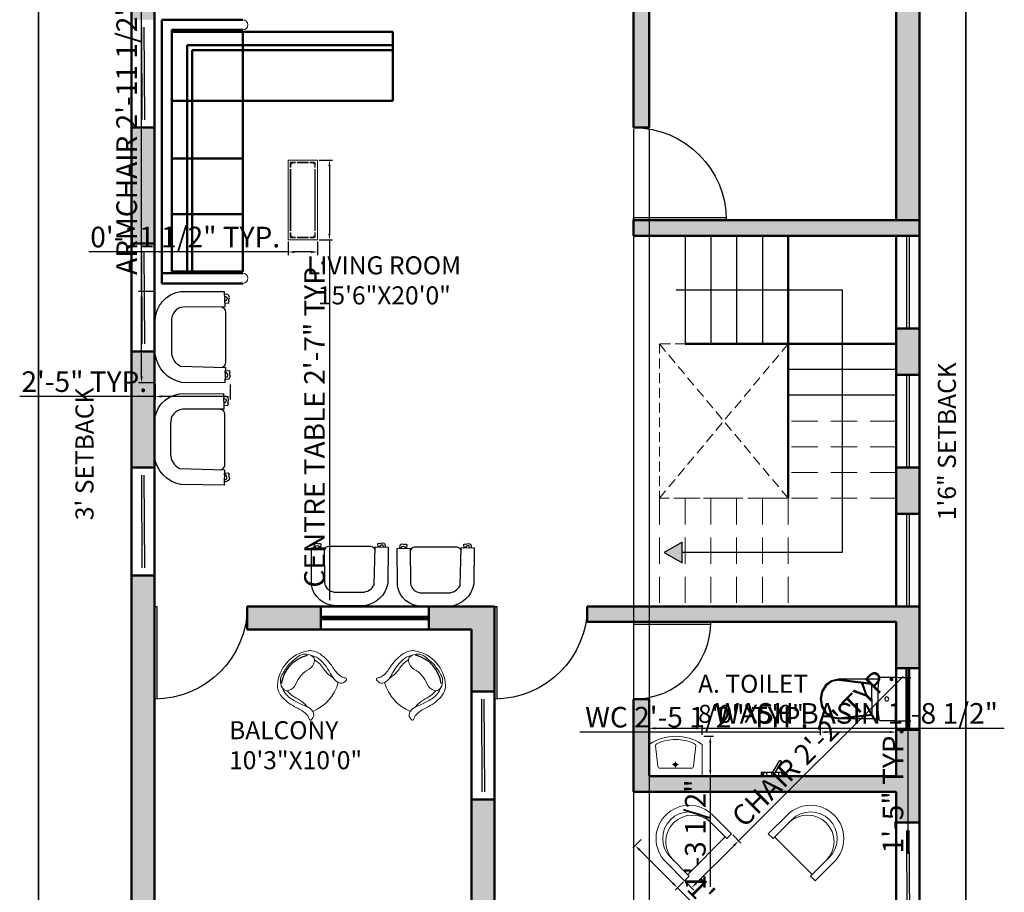
# Model space of a CAD drawing. Units: inches. Extents: x 1986 to 21484, y -1816 to 2016.
# Tile 42 of 85: x 2493 to 2875, y 1277 to 1616. Entities that reach past the tile are written whole.
import ezdxf

# ---------------------------------------------------------------- set-up
doc = ezdxf.new("R2010")
doc.units = ezdxf.units.IN
doc.linetypes.add('DASHED', pattern=[19.05, 12.7, -6.35])
for name, color, linetype in [('2D', 7, 'Continuous'), ('IFF-FURN-DETAIL', 250, 'Continuous'), ('SANTEH', 7, 'Continuous')]:
    doc.layers.add(name, color=color, linetype=linetype)
for name, color, linetype, lineweight in [('A-ANNO-DIMS', 2, 'Continuous', 18), ('A-ANNO-TEXT', 7, 'Continuous', 18), ('A-AREA-IDEN', 3, 'Continuous', 18), ('A-DOOR', 3, 'Continuous', 25), ('A-FLOR-FIXT', 8, 'Continuous', 18), ('A-FLOR-STRS', 7, 'Continuous', 25), ('A-FLOR-STRS-OVHD', 8, 'DASHED', 18), ('A-FURN', 8, 'Continuous', 18), ('A-GLAZ', 4, 'Continuous', 25), ('A-WALL', 7, 'Continuous', 50), ('A-WALL-PATT', 8, 'Continuous', 13), ('C-PROP', 7, 'Continuous', 35)]:
    doc.layers.add(name, color=color, linetype=linetype, lineweight=lineweight)
doc.styles.get("Standard").update_dxf_attribs({"font": 'arial.ttf'})
doc.dimstyles.new('ISO-25', dxfattribs={"dimtxt": 8, "dimasz": 2.5, "dimexe": 1.25, "dimexo": 0.625, "dimtad": 1, "dimdec": 1, "dimlunit": 3, "dimtxsty": 'Standard', "dimcen": 2.5, "dimadec": 0, "dimazin": 0, "dimtfac": 1, "dimtdec": 1, "dimtmove": 0, "dimatfit": 3, "dimfxl": 1, "dimarcsym": 0})

# ---------------------------------------------------------------- blocks, each defined once
blk = doc.blocks.new('D1')
for p, q in [((1805.96, 1500.36), (1805.96, 1464.36)), ((1806.96, 1500.36), (1806.96, 1464.36)), ((1805.96, 1464.36), (1806.96, 1464.36))]:
    blk.add_line(p, q)
blk.add_arc((1805.96, 1464.36), 36, 0, 90)
blk = doc.blocks.new('D2')
for p, q in [((1722.5, 1505.46), (1722.5, 1475.46)), ((1723.5, 1505.46), (1723.5, 1475.46)), ((1722.5, 1475.46), (1723.5, 1475.46))]:
    blk.add_line(p, q)
blk.add_arc((1722.5, 1475.46), 30, 0, 90)
blk = doc.blocks.new('WC 2 Symb_109')
at = {"layer": 'SANTEH'}
for p, q in [((0, 0), (0, 380)), ((0, 380), (132.4, 380)), ((153.6, 364.9), (506.8, 364.9)), ((506.3, 364.9), (215.7, 330.9)), ((506.3, 356), (215.7, 322)), ((215.7, 190), (215.7, 330.9)), ((215.7, 190), (215.7, 49.1)), ((153.8, 15.1), (506.8, 15.1)), ((506.3, 24), (215.7, 58)), ((506.3, 15.1), (215.7, 49.1)), ((0, 0), (132.4, 0))]:
    blk.add_line(p, q, dxfattribs=at)
for points in [[(154.6, 360.1), (153.9, 364.1), (152.3, 367.9), (150.2, 371.3), (147.4, 374.3), (144.1, 376.7), (140.5, 378.5), (136.5, 379.6), (132.4, 380)], [(154.6, 19.7), (158.6, 62.1), (161.4, 104.7), (163.1, 147.3), (163.7, 189.9), (163.1, 232.5), (161.4, 275.1), (158.6, 317.7), (154.6, 360.1)], [(506.3, 24), (565.5, 36.6), (615.7, 72.6), (649.2, 126.5), (661, 190), (649.2, 253.5), (615.7, 307.4), (565.5, 343.4), (506.3, 356)], [(506.8, 15.1), (569.2, 28.4), (622.2, 66.3), (657.6, 123.1), (670, 190), (657.6, 256.9), (622.2, 313.7), (569.2, 351.6), (506.8, 364.9)], [(132.4, 0), (136.5, 0.4), (140.4, 1.5), (144.1, 3.2), (147.3, 5.6), (150.1, 8.6), (152.3, 12), (153.8, 15.7), (154.6, 19.7)]]:
    blk.add_lwpolyline(points, dxfattribs=at)
blk.add_lwpolyline([(83.6, 208.5), (70.4, 203.1), (64.9, 190), (70.4, 176.9), (83.6, 171.5), (96.8, 176.9), (102.2, 190), (96.8, 203.1)], close=True, dxfattribs=at)
blk = doc.blocks.new('A$C2EBB240D')
for p, q in [((480, 375.8), (20, 375.8)), ((0, 355.8), (0, 86.6)), ((60.8, 89.8), (82.3, 282.2)), ((250, 300), (102.1, 300)), ((250, 300), (397.9, 300)), ((439.2, 89.8), (417.7, 282.2)), ((500, 355.8), (500, 86.6))]:
    blk.add_line(p, q)
for points in [[(247.3, 238.5), (247.3, 288.9)], [(275.2, 266.4), (219.4, 266.4)]]:
    blk.add_lwpolyline(points)
for centre, radius, start, end in [((20, 355.8), 20, 90, 180), ((480, 355.8), 20, 0, 90), ((102.1, 280), 20, 90, 173.64284), ((247.3, 266.4), 16.7, 90, 270), ((247.3, 266.4), 16.7, 270, 90), ((397.9, 280), 20, 6.35716, 90), ((247.3, 266.4), 10, 90, 270), ((247.3, 266.4), 10, 270, 90), ((20, 86.6), 20, 180, 237.68921), ((250, 450.3), 450.3, 237.68921, 270), ((80.7, 87.6), 20, 173.64284, 244.97956), ((250, 450.3), 420.3, 244.97956, 270), ((250, 450.3), 450.3, 270, 302.31079), ((250, 450.3), 420.3, 270, 295.02044), ((419.3, 87.6), 20, 295.02044, 6.35716), ((480, 86.6), 20, 302.31079, 0)]:
    blk.add_arc(centre, radius, start, end)
blk = doc.blocks.new('Faucet - kit sink top')
at = {"layer": 'SANTEH'}
for p, q in [((-5.5, -0.75), (-5.5, -1.25)), ((-4.94278, -0.75), (-5.5, -0.75)), ((-5.5, -1.25), (-4.94278, -1.25)), ((-0.14775, -1.7441), (3.56698, -8.1782)), ((4.43301, -7.6782), (0.71828, -1.2441)), ((4.94278, -0.75), (5.5, -0.75)), ((5.5, -1.25), (4.94278, -1.25)), ((5.5, -0.75), (5.5, -1.25))]:
    blk.add_line(p, q, dxfattribs=at)
blk.add_lwpolyline([(-0.00587, -2), (-6, -2), (-6, 0), (6, 0), (6, -2), (1.15195, -2)], dxfattribs=at)
for centre, radius in [((-4, -1), 1), ((4, -1), 1), ((0, -1), 0.75)]:
    blk.add_circle(centre, radius, dxfattribs=at)
blk.add_arc((4, -7.9282), 0.5, 210, 30, dxfattribs=at)
blk = doc.blocks.new('ILNG95')
for points in [[(120, 308, -0.32971), (51, 384, -0.036099), (50, 422, -0.497733), (75, 439, -0.070621), (96, 429, 0.101868), (133, 414, 0.091794), (259, 412, 0.024114), (351, 433, -0.090294), (638, 458, -0.132412), (775, 407, -0.068618), (816, 368, -0.184346), (943, 0, 1.803905)], [(120, 308, 0.138132), (244, 313, 0.001085), (325, 339, -0.034227), (462, 375, -0.033255), (567, 387, -0.137428), (727, 350, -4.561553)], [(120, 308, 0.138132), (244, 313, 0.001085), (325, 339, -0.034227), (462, 375, -0.033255), (567, 387, -0.137428), (727, 350, -4.561553)], [(235, 308, 0.064243), (394, 307, 0.04414), (433, 315, -0.118032), (643, 329, -6.296816)], [(235, 308, 0.064243), (394, 307, 0.04414), (433, 315, -0.118032), (643, 329, -6.296816)], [(639, 0, 0.078302), (612, 161, -0.233633), (633, 315, -0.28763), (710, 349, -0.317923), (875, 193, -0.032882), (900, 0, 1.140397)], [(639, 0, 0.078302), (612, 161, -0.233633), (633, 315, -0.28763), (710, 349, -0.317923), (875, 193, -0.032882), (900, 0, 1.140397)], [(120, -308, 0.32971), (51, -384, 0.036099), (50, -422, 0.497733), (75, -439, 0.070621), (96, -429, -0.101868), (133, -414, -0.091794), (259, -412, -0.024114), (351, -433, 0.090294), (638, -458, 0.132412), (775, -407, 0.068618), (816, -368, 0.184346), (943, 0, -1.803905)], [(639, 0, -0.078302), (612, -161, 0.233633), (633, -315, 0.28763), (710, -349, 0.317923), (875, -193, 0.032882), (900, 0, -1.140397)], [(639, 0, -0.078302), (612, -161, 0.233633), (633, -315, 0.28763), (710, -349, 0.317923), (875, -193, 0.032882), (900, 0, -1.140397)], [(120, -308, -0.138132), (244, -313, -0.001085), (325, -339, 0.034227), (462, -375, 0.033255), (567, -387, 0.137428), (727, -350, 4.561553)], [(120, -308, -0.138132), (244, -313, -0.001085), (325, -339, 0.034227), (462, -375, 0.033255), (567, -387, 0.137428), (727, -350, 4.561553)], [(235, -308, -0.064243), (394, -307, -0.04414), (433, -315, 0.118032), (643, -329, 6.296816)], [(235, -308, -0.064243), (394, -307, -0.04414), (433, -315, 0.118032), (643, -329, 6.296816)]]:
    blk.add_lwpolyline(points, format="xyb")
blk.add_arc((759, 1), 709, 154.3281, 205.801)
at = {"layer": 'IFF-FURN-DETAIL'}
blk.add_arc((326, -2), 549, 326.8997, 34.6691, dxfattribs=at)
blk.add_arc((326, -2), 549, 326.8997, 34.6691, dxfattribs=at)
blk = doc.blocks.new('12PSTG07')
at = {"color": 0, "linetype": 'ByBlock'}
for p, q in [((0, 15), (-12, 15)), ((0, 12), (0, 15)), ((-12, 12), (0, 12)), ((-1, -12), (-1, 12)), ((-12, -12), (0, -12)), ((0, -12), (0, -15)), ((0, -15), (-12, -15))]:
    blk.add_line(p, q, dxfattribs=at)
for centre, radius in [((-12, 0), 15), ((-12, 0), 12), ((-10, 0), 12)]:
    blk.add_arc(centre, radius, 90, 270, dxfattribs=at)
blk = doc.blocks.new('TABLE-30A')
at = {"color": 0, "linetype": 'ByBlock'}
for p, q in [((0, 0), (0, 0.55)), ((0, 0.55), (1.5, 0.55)), ((0.051, 0.508), (0.042, 0.499)), ((0.042, 0.499), (0.042, 0.478)), ((0.042, 0.478), (0.072, 0.478)), ((0.042, 0.478), (0.042, 0.41)), ((0.042, 0.169), (0.042, 0.381)), ((0.072, 0.508), (0.051, 0.508)), ((0.051, 0.478), (0.051, 0.41)), ((0.051, 0.169), (0.051, 0.381)), ((0.072, 0.478), (0.072, 0.508)), ((0.072, 0.508), (0.14, 0.508)), ((0.072, 0.499), (0.14, 0.499)), ((1.331, 0.508), (0.169, 0.508)), ((1.331, 0.499), (0.169, 0.499)), ((1.428, 0.508), (1.36, 0.508)), ((1.428, 0.499), (1.36, 0.499)), ((1.428, 0.508), (1.428, 0.478)), ((1.449, 0.508), (1.428, 0.508)), ((1.428, 0.478), (1.458, 0.478)), ((1.458, 0.499), (1.449, 0.508)), ((1.449, 0.478), (1.449, 0.41)), ((1.449, 0.381), (1.449, 0.169)), ((1.458, 0.478), (1.458, 0.499)), ((1.458, 0.478), (1.458, 0.41)), ((1.458, 0.381), (1.458, 0.169)), ((1.5, 0.55), (1.5, 0)), ((1.5, 0), (0, 0)), ((0.042, 0.072), (0.042, 0.14)), ((0.042, 0.072), (0.042, 0.051)), ((0.072, 0.072), (0.042, 0.072)), ((0.042, 0.051), (0.051, 0.042)), ((0.051, 0.072), (0.051, 0.14)), ((0.051, 0.042), (0.072, 0.042)), ((0.072, 0.042), (0.072, 0.072)), ((0.072, 0.051), (0.14, 0.051)), ((0.072, 0.042), (0.14, 0.042)), ((0.169, 0.051), (1.331, 0.051)), ((0.169, 0.042), (1.331, 0.042)), ((1.428, 0.051), (1.36, 0.051)), ((1.428, 0.042), (1.36, 0.042)), ((1.428, 0.072), (1.428, 0.042)), ((1.458, 0.072), (1.428, 0.072)), ((1.428, 0.042), (1.449, 0.042)), ((1.449, 0.072), (1.449, 0.14)), ((1.449, 0.042), (1.458, 0.051)), ((1.458, 0.072), (1.458, 0.14)), ((1.458, 0.051), (1.458, 0.072))]:
    blk.add_line(p, q, dxfattribs=at)
blk = doc.blocks.new('S 1')
at = {"layer": '2D'}
blk.add_lwpolyline([(4300.17, 1811.07), (4294.36, 1811.27), (4294.5, 1827.76, -0.326306), (4305.18, 1837.77), (4318.07, 1837.77, -0.372891), (4329.09, 1828.23), (4329.16, 1811.54), (4323.28, 1811.34), (4323.21, 1827.16, 0.399039), (4317.87, 1831.63), (4306.12, 1831.63, 0.288471), (4300.71, 1828.23)], format="xyb", close=True, dxfattribs=at)
for points in [[(4296.37, 1811.14), (4296.63, 1810.34), (4297.23, 1810.21), (4298.1, 1810.54), (4298.1, 1811.14), (4298.9, 1811.14), (4299.04, 1809.54), (4298.24, 1809.34), (4298.17, 1809.61), (4296.9, 1809.27), (4296.17, 1809.47), (4295.77, 1809.94), (4295.63, 1810.74), (4295.63, 1811.21)], [(4327.35, 1811.41), (4327.09, 1810.61), (4326.49, 1810.47), (4325.62, 1810.81), (4325.62, 1811.41), (4324.82, 1811.41), (4324.68, 1809.81), (4325.48, 1809.61), (4325.55, 1809.87), (4326.82, 1809.54), (4327.55, 1809.74), (4327.95, 1810.21), (4328.09, 1811.01), (4328.09, 1811.47)]]:
    blk.add_lwpolyline(points, dxfattribs=at)
blk.add_lwpolyline([(4300.24, 1812.34, 0.33845), (4302.18, 1810.94), (4321.28, 1810.94, 0.381322), (4323.15, 1812.61, -0.892406)], format="xyb", dxfattribs=at)
blk = doc.blocks.new('WIN-36')
for p, q in [((0, 36), (0, 0)), ((0, 36), (0, 0)), ((1, 36), (1, 0))]:
    blk.add_line(p, q)
blk = doc.blocks.new('*D97')
at = {"layer": 'A-ANNO-DIMS', "color": 0, "lineweight": -2, "transparency": 16777216}
for p, q in [((2803.7, 1342.73), (2803.7, 1337.67)), ((2833.31, 1342.73), (2833.31, 1337.67)), ((2803.7, 1338.92), (2710.49, 1338.92)), ((2830.81, 1338.92), (2806.2, 1338.92))]:
    blk.add_line(p, q, dxfattribs=at)
at = {"layer": 'A-ANNO-DIMS', "color": 0, "transparency": 16777216}
for points in [[(2806.2, 1339.33), (2806.2, 1338.5), (2803.7, 1338.92)], [(2830.81, 1339.33), (2830.81, 1338.5), (2833.31, 1338.92)]]:
    blk.add_solid(points, dxfattribs=at)
at = {"layer": 'Defpoints', "color": 0, "transparency": 16777216}
for p in [(2803.7, 1343.36), (2833.31, 1343.36), (2803.7, 1338.92)]:
    blk.add_point(p, dxfattribs=at)
at = {"layer": 'A-ANNO-DIMS', "color": 0, "transparency": 16777216, "insert": (2755.85, 1343.68), "char_height": 8, "attachment_point": 5}
blk.add_mtext('WC 2\'-5 1/2" TYP.', dxfattribs=at)
blk = doc.blocks.new('*D98')
at = {"layer": 'A-ANNO-DIMS', "color": 0, "lineweight": -2, "transparency": 16777216}
for p, q in [((2833.93, 1360.15), (2839, 1360.15)), ((2837.75, 1357.65), (2837.75, 1345.86)), ((2833.93, 1343.36), (2839, 1343.36)), ((2837.75, 1343.36), (2837.75, 1291.6))]:
    blk.add_line(p, q, dxfattribs=at)
at = {"layer": 'A-ANNO-DIMS', "color": 0, "transparency": 16777216}
for points in [[(2837.33, 1357.65), (2838.16, 1357.65), (2837.75, 1360.15)], [(2837.33, 1345.86), (2838.16, 1345.86), (2837.75, 1343.36)]]:
    blk.add_solid(points, dxfattribs=at)
at = {"layer": 'Defpoints', "color": 0, "transparency": 16777216}
for p in [(2833.31, 1360.15), (2833.31, 1343.36), (2837.75, 1343.36)]:
    blk.add_point(p, dxfattribs=at)
at = {"layer": 'A-ANNO-DIMS', "color": 0, "transparency": 16777216, "insert": (2833.04, 1316.23), "char_height": 8, "attachment_point": 5, "rotation": 90}
blk.add_mtext('1\'-5" TYP.', dxfattribs=at)
blk = doc.blocks.new('*D99')
at = {"layer": 'A-ANNO-DIMS', "color": 0, "lineweight": -2, "transparency": 16777216}
for p, q in [((2737.31, 1337.91), (2737.31, 1341.64)), ((2739.81, 1340.39), (2755.48, 1340.39)), ((2757.98, 1337.91), (2757.98, 1341.64)), ((2757.98, 1340.39), (2875.24, 1340.39))]:
    blk.add_line(p, q, dxfattribs=at)
at = {"layer": 'A-ANNO-DIMS', "color": 0, "transparency": 16777216}
for points in [[(2739.81, 1340.81), (2739.81, 1339.97), (2737.31, 1340.39)], [(2755.48, 1340.81), (2755.48, 1339.97), (2757.98, 1340.39)]]:
    blk.add_solid(points, dxfattribs=at)
at = {"layer": 'Defpoints', "color": 0, "transparency": 16777216}
for p in [(2757.98, 1340.39), (2737.31, 1337.29), (2757.98, 1337.29)]:
    blk.add_point(p, dxfattribs=at)
at = {"layer": 'A-ANNO-DIMS', "color": 0, "transparency": 16777216, "insert": (2817.86, 1345.15), "char_height": 8, "attachment_point": 5}
blk.add_mtext('WASH BASIN 1\'-8 1/2"', dxfattribs=at)
blk = doc.blocks.new('*D100')
at = {"layer": 'A-ANNO-DIMS', "color": 0, "lineweight": -2, "transparency": 16777216}
for p, q in [((2758.6, 1337.29), (2762.33, 1337.29)), ((2761.08, 1334.79), (2761.08, 1324.25)), ((2758.6, 1321.75), (2762.33, 1321.75)), ((2761.08, 1321.75), (2761.08, 1278.85))]:
    blk.add_line(p, q, dxfattribs=at)
at = {"layer": 'A-ANNO-DIMS', "color": 0, "transparency": 16777216}
for points in [[(2760.66, 1334.79), (2761.5, 1334.79), (2761.08, 1337.29)], [(2760.66, 1324.25), (2761.5, 1324.25), (2761.08, 1321.75)]]:
    blk.add_solid(points, dxfattribs=at)
at = {"layer": 'Defpoints', "color": 0, "transparency": 16777216}
for p in [(2757.98, 1337.29), (2757.98, 1321.75), (2761.08, 1321.75)]:
    blk.add_point(p, dxfattribs=at)
at = {"layer": 'A-ANNO-DIMS', "color": 0, "transparency": 16777216, "insert": (2756.31, 1299.05), "char_height": 8, "attachment_point": 5, "rotation": 90}
blk.add_mtext('1\'-3 1/2"', dxfattribs=at)
blk = doc.blocks.new('*D103')
at = {"layer": 'A-ANNO-DIMS', "color": 0, "lineweight": -2, "transparency": 16777216}
for p, q in [((2772.08, 1296.67), (2835.93, 1360.53)), ((2769.78, 1298.97), (2772.96, 1295.79)), ((2755.61, 1280.2), (2770.31, 1294.91)), ((2751.54, 1280.73), (2754.72, 1277.55))]:
    blk.add_line(p, q, dxfattribs=at)
at = {"layer": 'A-ANNO-DIMS', "color": 0, "transparency": 16777216}
for points in [[(2770.01, 1295.2), (2770.6, 1294.61), (2772.08, 1296.67)], [(2755.31, 1280.5), (2755.9, 1279.91), (2753.84, 1278.44)]]:
    blk.add_solid(points, dxfattribs=at)
at = {"layer": 'Defpoints', "color": 0, "transparency": 16777216}
for p in [(2769.34, 1299.41), (2772.08, 1296.67), (2751.1, 1281.17)]:
    blk.add_point(p, dxfattribs=at)
at = {"layer": 'A-ANNO-DIMS', "color": 0, "transparency": 16777216, "insert": (2801.52, 1332.85), "char_height": 8, "attachment_point": 5, "rotation": 45}
blk.add_mtext('CHAIR 2\'-2" TYP.', dxfattribs=at)
blk = doc.blocks.new('*D104')
at = {"layer": 'A-ANNO-DIMS', "color": 0, "lineweight": -2, "transparency": 16777216}
for p, q in [((2734.24, 1297.14), (2731.07, 1293.97)), ((2733.72, 1293.08), (2746.6, 1280.2)), ((2750.66, 1280.73), (2747.48, 1277.55)), ((2748.37, 1278.44), (2789.36, 1237.44))]:
    blk.add_line(p, q, dxfattribs=at)
at = {"layer": 'A-ANNO-DIMS', "color": 0, "transparency": 16777216}
for points in [[(2734.01, 1293.38), (2733.42, 1292.79), (2731.95, 1294.85)], [(2746.89, 1280.5), (2746.3, 1279.91), (2748.37, 1278.44)]]:
    blk.add_solid(points, dxfattribs=at)
at = {"layer": 'Defpoints', "color": 0, "transparency": 16777216}
for p in [(2734.69, 1297.59), (2751.1, 1281.17), (2748.37, 1278.44)]:
    blk.add_point(p, dxfattribs=at)
at = {"layer": 'A-ANNO-DIMS', "color": 0, "transparency": 16777216, "insert": (2773.03, 1260.34), "char_height": 8, "attachment_point": 5, "rotation": 315}
blk.add_mtext('1\'-11" TYP.', dxfattribs=at)
blk = doc.blocks.new('*D109')
at = {"layer": 'A-ANNO-DIMS', "color": 0, "lineweight": -2, "transparency": 16777216}
for p, q in [((2540.28, 1510.13), (2540.28, 1650.68)), ((2544.98, 1510.13), (2539.03, 1510.13)), ((2540.28, 1477.15), (2540.28, 1507.63)), ((2544.98, 1474.65), (2539.03, 1474.65))]:
    blk.add_line(p, q, dxfattribs=at)
at = {"layer": 'A-ANNO-DIMS', "color": 0, "transparency": 16777216}
for points in [[(2539.86, 1507.63), (2540.7, 1507.63), (2540.28, 1510.13)], [(2539.86, 1477.15), (2540.7, 1477.15), (2540.28, 1474.65)]]:
    blk.add_solid(points, dxfattribs=at)
at = {"layer": 'Defpoints', "color": 0, "transparency": 16777216}
for p in [(2540.28, 1510.13), (2545.6, 1510.13), (2545.6, 1474.65)]:
    blk.add_point(p, dxfattribs=at)
at = {"layer": 'A-ANNO-DIMS', "color": 0, "transparency": 16777216, "insert": (2535.52, 1581.65), "char_height": 8, "attachment_point": 5, "rotation": 90}
blk.add_mtext('ARMCHAIR 2\'-11 1/2" TYP.', dxfattribs=at)
blk = doc.blocks.new('*D110')
at = {"layer": 'A-ANNO-DIMS', "color": 0, "lineweight": -2, "transparency": 16777216}
for p, q in [((2545.6, 1474.02), (2545.6, 1468.07)), ((2574.67, 1474.02), (2574.67, 1468.07)), ((2545.6, 1469.32), (2492.95, 1469.32)), ((2572.17, 1469.32), (2548.1, 1469.32))]:
    blk.add_line(p, q, dxfattribs=at)
at = {"layer": 'A-ANNO-DIMS', "color": 0, "transparency": 16777216}
for points in [[(2548.1, 1469.74), (2548.1, 1468.91), (2545.6, 1469.32)], [(2572.17, 1469.74), (2572.17, 1468.91), (2574.67, 1469.32)]]:
    blk.add_solid(points, dxfattribs=at)
at = {"layer": 'Defpoints', "color": 0, "transparency": 16777216}
for p in [(2545.6, 1474.65), (2574.67, 1474.65), (2545.6, 1469.32)]:
    blk.add_point(p, dxfattribs=at)
at = {"layer": 'A-ANNO-DIMS', "color": 0, "transparency": 16777216, "insert": (2518.03, 1474.03), "char_height": 8, "attachment_point": 5}
blk.add_mtext('2\'-5" TYP.', dxfattribs=at)
blk = doc.blocks.new('*D111')
at = {"layer": 'A-ANNO-DIMS', "color": 0, "lineweight": -2, "transparency": 16777216}
for p, q in [((2609.17, 1561.17), (2614.46, 1561.17)), ((2613.21, 1558.67), (2613.21, 1532.6)), ((2609.17, 1530.1), (2614.46, 1530.1)), ((2613.21, 1530.1), (2613.21, 1390.12))]:
    blk.add_line(p, q, dxfattribs=at)
at = {"layer": 'A-ANNO-DIMS', "color": 0, "transparency": 16777216}
for points in [[(2612.79, 1558.67), (2613.62, 1558.67), (2613.21, 1561.17)], [(2612.79, 1532.6), (2613.62, 1532.6), (2613.21, 1530.1)]]:
    blk.add_solid(points, dxfattribs=at)
at = {"layer": 'Defpoints', "color": 0, "transparency": 16777216}
for p in [(2608.55, 1561.17), (2608.55, 1530.1), (2613.21, 1530.1)]:
    blk.add_point(p, dxfattribs=at)
at = {"layer": 'A-ANNO-DIMS', "color": 0, "transparency": 16777216, "insert": (2608.44, 1458.86), "char_height": 8, "attachment_point": 5, "rotation": 90}
blk.add_mtext('CENTRE TABLE 2\'-7" TYP.', dxfattribs=at)
blk = doc.blocks.new('*D112')
at = {"layer": 'A-ANNO-DIMS', "color": 0, "lineweight": -2, "transparency": 16777216}
for p, q in [((2597.16, 1529.48), (2597.16, 1524.19)), ((2608.55, 1529.48), (2608.55, 1524.19)), ((2597.16, 1525.44), (2519.79, 1525.44)), ((2606.05, 1525.44), (2599.66, 1525.44))]:
    blk.add_line(p, q, dxfattribs=at)
at = {"layer": 'A-ANNO-DIMS', "color": 0, "transparency": 16777216}
for points in [[(2599.66, 1525.86), (2599.66, 1525.03), (2597.16, 1525.44)], [(2606.05, 1525.86), (2606.05, 1525.03), (2608.55, 1525.44)]]:
    blk.add_solid(points, dxfattribs=at)
at = {"layer": 'Defpoints', "color": 0, "transparency": 16777216}
for p in [(2597.16, 1530.1), (2608.55, 1530.1), (2597.16, 1525.44)]:
    blk.add_point(p, dxfattribs=at)
at = {"layer": 'A-ANNO-DIMS', "color": 0, "transparency": 16777216, "insert": (2557.22, 1530.21), "char_height": 8, "attachment_point": 5}
blk.add_mtext('0\'-11 1/2" TYP.', dxfattribs=at)
blk = doc.blocks.new('*D137')
at = {"layer": 'A-ANNO-DIMS', "color": 0, "lineweight": -2, "transparency": 16777216}
for p, q in [((2731.31, 1573.13), (2731.31, 953.11)), ((2737.31, 1573.13), (2737.31, 953.11)), ((2728.81, 954.36), (2726.31, 954.36)), ((2731.31, 954.36), (2737.31, 954.36)), ((2739.81, 954.36), (2764.82, 954.36))]:
    blk.add_line(p, q, dxfattribs=at)
at = {"layer": 'A-ANNO-DIMS', "color": 0, "transparency": 16777216}
for points in [[(2728.81, 954.78), (2728.81, 953.95), (2731.31, 954.36)], [(2739.81, 954.78), (2739.81, 953.95), (2737.31, 954.36)]]:
    blk.add_solid(points, dxfattribs=at)
at = {"layer": 'Defpoints', "color": 0, "transparency": 16777216}
for p in [(2731.31, 1573.75), (2737.31, 1573.75), (2737.31, 954.36)]:
    blk.add_point(p, dxfattribs=at)
at = {"layer": 'A-ANNO-DIMS', "color": 0, "transparency": 16777216, "insert": (2753.56, 959.07), "char_height": 8, "attachment_point": 5}
blk.add_mtext('0\'-6"', dxfattribs=at)

msp = doc.modelspace()

# ---------------------------------------------------------------- hatches: boundary and pattern name
at = {"layer": 'A-FLOR-STRS'}
h = msp.add_hatch(color=256, dxfattribs=at)
h.dxf.hatch_style = 1
h.paths.add_polyline_path([(2743.15, 1408.75), (2750.1, 1404.74), (2750.1, 1412.77)])
at = {"layer": 'A-WALL-PATT'}
h = msp.add_hatch(color=256, dxfattribs=at)
h.dxf.hatch_style = 1
h.paths.add_polyline_path([(2545.31, 1843.75), (2665.31, 1843.75), (2665.31, 1852.75), (2536.31, 1852.75), (2536.31, 1765.75), (2545.31, 1765.75)])
h.paths.add_polyline_path([(2545.31, 1723.75), (2536.31, 1723.75), (2536.31, 1675.75), (2545.31, 1675.75), (2545.31, 1693.75), (2629.31, 1693.75), (2629.31, 1681.75), (2635.31, 1681.75), (2635.31, 1693.75), (2641.31, 1693.75), (2641.31, 1699.75), (2545.31, 1699.75)])
h.paths.add_polyline_path([(2545.31, 1651.75), (2536.31, 1651.75), (2536.31, 1615.75), (2545.31, 1615.75), (2545.31, 1627.75), (2695.31, 1627.75), (2695.31, 1699.75), (2671.31, 1699.75), (2671.31, 1693.75), (2689.31, 1693.75), (2689.31, 1633.75), (2635.31, 1633.75), (2635.31, 1651.75), (2629.31, 1651.75), (2629.31, 1633.75), (2545.31, 1633.75)])
h.paths.add_polyline_path([(2545.31, 1573.75), (2536.31, 1573.75), (2536.31, 1528.77), (2545.31, 1528.77)])
h.paths.add_polyline_path([(2545.31, 1486.77), (2536.31, 1486.77), (2536.31, 1441.75), (2545.31, 1441.75)])
h.paths.add_polyline_path([(2545.31, 1399.75), (2536.31, 1399.75), (2536.31, 1258.75), (2545.31, 1258.75)])
h.paths.add_polyline_path([(2609.81, 1387.75), (2581.31, 1387.75), (2581.31, 1378.75), (2609.81, 1378.75)])
h.paths.add_polyline_path([(2677.31, 1387.75), (2651.81, 1387.75), (2651.81, 1378.75), (2668.31, 1378.75), (2668.31, 1354.75), (2677.31, 1354.75)])
h.paths.add_polyline_path([(2842.31, 1387.75), (2833.31, 1387.75), (2713.31, 1387.75), (2713.31, 1381.75), (2833.31, 1381.75), (2833.31, 1363.75), (2842.31, 1363.75)])
h.paths.add_polyline_path([(2842.31, 1339.75), (2833.31, 1339.75), (2833.31, 1321.75), (2737.31, 1321.75), (2737.31, 1351.75), (2731.31, 1351.75), (2731.31, 1315.75), (2833.31, 1315.75), (2833.31, 1303.75), (2842.31, 1303.75)])
h.paths.add_polyline_path([(2677.31, 1312.75), (2668.31, 1312.75), (2668.31, 1189.75), (2677.31, 1189.75)])
h.paths.add_polyline_path([(2677.31, 1147.75), (2668.31, 1147.75), (2668.31, 1114.75), (2683.31, 1114.75), (2683.31, 1123.75), (2677.31, 1123.75)])
h.paths.add_polyline_path([(2842.31, 1147.75), (2833.31, 1147.75), (2833.31, 1123.75), (2725.31, 1123.75), (2725.31, 1114.75), (2842.31, 1114.75)])
h.paths.add_polyline_path([(2842.31, 1261.75), (2833.31, 1261.75), (2833.31, 1189.75), (2842.31, 1189.75)])
h.paths.add_polyline_path([(2842.31, 1441.75), (2833.31, 1441.75), (2833.31, 1423.75), (2842.31, 1423.75)])
h.paths.add_polyline_path([(2842.31, 1495.75), (2833.31, 1495.75), (2833.31, 1477.75), (2842.31, 1477.75)])
h.paths.add_polyline_path([(2737.31, 1852.75), (2707.31, 1852.75), (2707.31, 1843.75), (2731.31, 1843.75), (2731.31, 1573.75), (2737.31, 1573.75)])
h.paths.add_polyline_path([(2719.29, 1802.81), (2719.29, 1755.53), (2727.83, 1755.53), (2727.83, 1802.81)], flags=25)
h.paths.add_polyline_path([(2682.04, 1129.8), (2724.23, 1129.8), (2724.23, 1138.34), (2682.04, 1138.34)], flags=9)
h.paths.add_polyline_path([(2763.84, 1129.8), (2811.12, 1129.8), (2811.12, 1138.34), (2763.84, 1138.34)], flags=25)
h.paths.add_polyline_path([(2759.39, 1682.81), (2810.29, 1682.81), (2810.29, 1709.43), (2759.39, 1709.43)], flags=9)
h.paths.add_polyline_path([(2636.77, 1656.28), (2690.81, 1656.28), (2690.81, 1682.89), (2636.77, 1682.89)], flags=25)
h.paths.add_polyline_path([(2525.6, 1419.09), (2525.6, 1479.38), (2510.65, 1479.38), (2510.65, 1419.09)], flags=9)
h.paths.add_polyline_path([(2860.43, 1418.3), (2860.43, 1487.98), (2845.48, 1487.98), (2845.48, 1418.3)], flags=9)
h.paths.add_polyline_path([(2725.63, 1084.99), (2785.92, 1084.99), (2785.92, 1099.93), (2725.63, 1099.93)], flags=9)
h.paths.add_polyline_path([(2602.46, 1501.1), (2675.15, 1501.1), (2675.15, 1527.71), (2602.46, 1527.71)], flags=9)
h.paths.add_polyline_path([(2571.3, 1320.51), (2625.79, 1320.51), (2625.79, 1347.12), (2571.3, 1347.12)], flags=9)
h.paths.add_polyline_path([(2729.91, 1208.98), (2797.91, 1208.98), (2797.91, 1235.59), (2729.91, 1235.59)], flags=9)
h.paths.add_polyline_path([(2753.97, 1338.54), (2806.8, 1338.54), (2806.8, 1365.15), (2753.97, 1365.15)], flags=9)
h.paths.add_polyline_path([(2605.23, 1760.02), (2661.46, 1760.02), (2661.46, 1786.64), (2605.23, 1786.64)], flags=9)
h.paths.add_polyline_path([(2558.03, 1656.28), (2610.63, 1656.28), (2610.63, 1682.89), (2558.03, 1682.89)], flags=25)
h = msp.add_hatch(color=256, dxfattribs=at)
h.dxf.hatch_style = 1
h.paths.add_polyline_path([(2842.31, 1852.75), (2737.31, 1852.75), (2737.31, 1843.75), (2833.31, 1843.75), (2833.31, 1537.75), (2842.31, 1537.75)])
h.paths.add_polyline_path([(2682.04, 1129.8), (2724.23, 1129.8), (2724.23, 1138.34), (2682.04, 1138.34)], flags=9)
h.paths.add_polyline_path([(2763.84, 1129.8), (2811.12, 1129.8), (2811.12, 1138.34), (2763.84, 1138.34)], flags=9)
h.paths.add_polyline_path([(2719.29, 1802.81), (2719.29, 1755.53), (2727.83, 1755.53), (2727.83, 1802.81)], flags=9)
h.paths.add_polyline_path([(2759.39, 1682.81), (2810.29, 1682.81), (2810.29, 1709.43), (2759.39, 1709.43)], flags=25)
h.paths.add_polyline_path([(2636.77, 1656.28), (2690.81, 1656.28), (2690.81, 1682.89), (2636.77, 1682.89)], flags=9)
h.paths.add_polyline_path([(2525.6, 1419.09), (2525.6, 1479.38), (2510.65, 1479.38), (2510.65, 1419.09)], flags=9)
h.paths.add_polyline_path([(2860.43, 1418.3), (2860.43, 1487.98), (2845.48, 1487.98), (2845.48, 1418.3)], flags=9)
h.paths.add_polyline_path([(2725.63, 1084.99), (2785.92, 1084.99), (2785.92, 1099.93), (2725.63, 1099.93)], flags=9)
h.paths.add_polyline_path([(2602.46, 1501.1), (2675.15, 1501.1), (2675.15, 1527.71), (2602.46, 1527.71)], flags=9)
h.paths.add_polyline_path([(2571.3, 1320.51), (2625.79, 1320.51), (2625.79, 1347.12), (2571.3, 1347.12)], flags=9)
h.paths.add_polyline_path([(2710.58, 1210.46), (2778.57, 1210.46), (2778.57, 1237.07), (2710.58, 1237.07)], flags=9)
h.paths.add_polyline_path([(2753.97, 1338.54), (2806.8, 1338.54), (2806.8, 1365.15), (2753.97, 1365.15)], flags=9)
h.paths.add_polyline_path([(2605.23, 1728.88), (2661.46, 1728.88), (2661.46, 1755.49), (2605.23, 1755.49)], flags=9)
h.paths.add_polyline_path([(2558.03, 1656.28), (2610.63, 1656.28), (2610.63, 1682.89), (2558.03, 1682.89)], flags=9)
h = msp.add_hatch(color=256, dxfattribs=at)
h.dxf.hatch_style = 1
h.paths.add_polyline_path([(2842.31, 1537.75), (2731.31, 1537.75), (2731.31, 1531.75), (2833.31, 1531.75), (2842.31, 1531.75)])

# ---------------------------------------------------------------- linework, layer by layer
at = {"layer": 'A-FLOR-STRS'}
for p, q in [((2751.31, 1531.75), (2751.31, 1489.75)), ((2761.31, 1531.75), (2761.31, 1489.75)), ((2771.31, 1531.75), (2771.31, 1489.75)), ((2781.31, 1531.75), (2781.31, 1489.75)), ((2833.31, 1479.75), (2791.31, 1479.75)), ((2833.31, 1469.75), (2791.31, 1469.75))]:
    msp.add_line(p, q, dxfattribs=at)
msp.add_lwpolyline([(2747.89, 1510.75), (2812.31, 1510.75), (2812.31, 1408.75), (2750.1, 1408.75)], dxfattribs=at)
msp.add_lwpolyline([(2743.15, 1408.75), (2750.1, 1404.74), (2750.1, 1412.77)], close=True, dxfattribs=at)
at = {"layer": 'A-FLOR-STRS-OVHD', "ltscale": 0.3}
for p, q in [((2741.31, 1489.75), (2791.31, 1429.75)), ((2741.31, 1429.75), (2791.31, 1489.75))]:
    msp.add_line(p, q, dxfattribs=at)
at = {"layer": 'A-FLOR-STRS-OVHD', "ltscale": 0.8}
for p, q in [((2833.31, 1459.75), (2791.31, 1459.75)), ((2833.31, 1449.75), (2791.31, 1449.75)), ((2833.31, 1439.75), (2791.31, 1439.75)), ((2741.31, 1429.75), (2741.31, 1387.75)), ((2833.31, 1429.75), (2741.31, 1429.75)), ((2751.31, 1429.75), (2751.31, 1387.75)), ((2761.31, 1429.75), (2761.31, 1387.75)), ((2771.31, 1429.75), (2771.31, 1387.75)), ((2781.31, 1429.75), (2781.31, 1387.75)), ((2791.31, 1429.75), (2791.31, 1387.75))]:
    msp.add_line(p, q, dxfattribs=at)
at = {"layer": 'A-FLOR-STRS-OVHD', "ltscale": 0.3}
msp.add_lwpolyline([(2741.31, 1429.75), (2791.31, 1429.75), (2791.31, 1489.75), (2741.31, 1489.75)], close=True, dxfattribs=at)
at = {"layer": 'A-FURN'}
for centre in [(2579.61, 1613.65), (2579.61, 1515.23)]:
    msp.add_arc(centre, 1.97, 270, 90, dxfattribs=at)
at = {"layer": 'A-WALL'}
for p, q in [((2536.31, 1258.75), (2536.31, 1852.75)), ((2737.31, 1852.75), (2737.31, 1573.75)), ((2842.31, 1852.75), (2842.31, 1114.75)), ((2731.31, 1843.75), (2731.31, 1573.75)), ((2833.31, 1843.75), (2833.31, 1537.75)), ((2545.31, 1258.75), (2545.31, 1627.75)), ((2548.11, 1615.62), (2548.11, 1513.26)), ((2579.61, 1615.62), (2548.11, 1615.62)), ((2552.05, 1611.69), (2552.05, 1517.85)), ((2579.61, 1611.69), (2552.05, 1611.69)), ((2552.05, 1611.03), (2637.84, 1611.03)), ((2579.61, 1517.85), (2579.61, 1611.03)), ((2637.84, 1611.03), (2637.84, 1584.13)), ((2557.96, 1605.78), (2557.96, 1517.85)), ((2637.84, 1605.78), (2557.96, 1605.78)), ((2559.92, 1603.81), (2559.92, 1517.85)), ((2637.84, 1603.81), (2559.92, 1603.81)), ((2552.05, 1584.13), (2637.84, 1584.13)), ((2574.36, 1584.13), (2637.84, 1584.13)), ((2536.31, 1573.75), (2545.31, 1573.75)), ((2731.31, 1573.75), (2737.31, 1573.75)), ((2552.05, 1561.82), (2579.61, 1561.82)), ((2552.05, 1540.16), (2579.61, 1540.16)), ((2731.31, 1537.75), (2842.31, 1537.75)), ((2731.31, 1537.75), (2731.31, 1531.75)), ((2731.31, 1531.75), (2833.31, 1531.75)), ((2791.31, 1531.75), (2791.31, 1429.75)), ((2833.31, 1531.75), (2833.31, 1387.75)), ((2833.31, 1531.75), (2842.31, 1531.75)), ((2536.31, 1528.77), (2545.31, 1528.77)), ((2552.05, 1517.85), (2579.61, 1517.85)), ((2548.11, 1517.2), (2579.61, 1517.2)), ((2548.11, 1513.26), (2579.61, 1513.26)), ((2833.31, 1495.75), (2842.31, 1495.75)), ((2833.31, 1489.75), (2751.31, 1489.75)), ((2536.31, 1486.77), (2545.31, 1486.77)), ((2833.31, 1477.75), (2842.31, 1477.75)), ((2536.31, 1441.75), (2545.31, 1441.75)), ((2833.31, 1441.75), (2842.31, 1441.75)), ((2833.31, 1423.75), (2842.31, 1423.75)), ((2536.31, 1399.75), (2545.31, 1399.75)), ((2581.31, 1378.75), (2581.31, 1387.75)), ((2581.31, 1387.75), (2677.31, 1387.75)), ((2609.81, 1378.75), (2609.81, 1387.75)), ((2651.81, 1378.75), (2651.81, 1387.75)), ((2677.31, 1123.75), (2677.31, 1387.75)), ((2713.31, 1387.75), (2833.31, 1387.75)), ((2713.31, 1381.75), (2713.31, 1387.75)), ((2833.31, 1387.75), (2842.31, 1387.75)), ((2609.81, 1383.75), (2651.81, 1383.75)), ((2609.81, 1382.75), (2651.81, 1382.75)), ((2713.31, 1381.75), (2833.31, 1381.75)), ((2833.31, 1381.75), (2833.31, 1321.75)), ((2581.31, 1378.75), (2668.31, 1378.75)), ((2668.31, 1114.75), (2668.31, 1378.75)), ((2833.31, 1363.75), (2842.31, 1363.75)), ((2837.31, 1339.75), (2837.31, 1363.75)), ((2838.31, 1339.75), (2838.31, 1363.75)), ((2668.31, 1354.75), (2677.31, 1354.75)), ((2731.31, 1351.75), (2731.31, 1315.75)), ((2731.31, 1351.75), (2737.31, 1351.75)), ((2737.31, 1351.75), (2737.31, 1321.75)), ((2833.31, 1339.75), (2842.31, 1339.75)), ((2737.31, 1321.75), (2833.31, 1321.75)), ((2731.31, 1315.75), (2833.31, 1315.75)), ((2833.31, 1315.75), (2833.31, 1123.75)), ((2668.31, 1312.75), (2677.31, 1312.75)), ((2833.31, 1303.75), (2842.31, 1303.75))]:
    msp.add_line(p, q, dxfattribs=at)
at = {"layer": 'C-PROP'}
msp.add_lwpolyline([(2500.31, 1900.75), (2860.31, 1900.75), (2860.31, 1066.75), (2500.31, 1066.75)], close=True, dxfattribs=at)

# ---------------------------------------------------------------- block references
at = {"layer": 'A-DOOR', "xscale": -1}
for p, rotation in [((1266.95, -268.21), 270), ((739.34, 2852.11), 180), ((871.34, 2852.11), 180)]:
    msp.add_blockref('D1', p, dxfattribs=dict(at, rotation=rotation))
at = {"layer": 'A-DOOR', "rotation": 270}
msp.add_blockref('D2', (1255.85, 3104.25), dxfattribs=at)
at = {"layer": 'A-FLOR-FIXT'}
for name, p, xscale, yscale, zscale, rotation in [('WC 2 Symb_109', (2833.31, 1360.15), 0.0441898926459964, 0.0441898926459964, 0.0441898926459964, 180), ('A$C2EBB240D', (2737.31, 1337.29), -0.0413429615335577, 0.0413429615335577, 0.0413429615335577, 180), ('Faucet - kit sink top', (2785.31, 1321.75), -0.7356136897818673, 0.7356136897818673, 0.7356136897818673, 180), ('12PSTG07', (2760.22, 1290.29), 0.8597921787217943, 0.8597921787217943, 0.8597921787217943, 315), ('12PSTG07', (2792.73, 1290.29), -0.8597921787217945, 0.8597921787217943, 0.8597921787217943, 45)]:
    msp.add_blockref(name, p, dxfattribs=dict(at, xscale=xscale, yscale=yscale, zscale=zscale, rotation=rotation))
at = {"layer": 'A-FURN'}
for name, p, xscale, yscale, zscale, rotation in [('TABLE-30A', (2608.55, 1561.17), -20.70834898381633, 20.70834898381633, 20.70834898381633, 90), ('S 1', (4419.78, -2904.78), 1.019808145295116, 1.019808145295116, 1.019808145295116, 89.99999999999999), ('S 1', (4419.46, -2944.51), 1.019808145295116, 1.019808145295116, 1.019808145295116, 89.99999999999999), ('S 1', (6313.3, 2961.73), 0.8563117011609614, 0.8563117011609614, 0.8563117011609614, 180), ('S 1', (6346.66, 2961.46), 0.8563117011609614, 0.8563117011609614, 0.8563117011609614, 180), ('ILNG95', (2613.89, 1350.61), -0.0243705291132055, 0.0243705291132055, 0.0243705291132055, 318.5881218623716), ('ILNG95', (2637.41, 1350.61), 0.0243705291132055, 0.0243705291132055, 0.0243705291132055, 41.41187813762839)]:
    msp.add_blockref(name, p, dxfattribs=dict(at, xscale=xscale, yscale=yscale, zscale=zscale, rotation=rotation))
at = {"layer": 'A-GLAZ'}
for p, rotation in [((2540.4, 1576.75), 0.3027934322096833), ((2540.4, 1489.77), 0.3027934322096833), ((2540.4, 1402.75), 0.302793432207276), ((2672.4, 1315.75), 0.302793432207276), ((2837.4, 1264.75), 0.302793432207276)]:
    msp.add_blockref('WIN-36', p, dxfattribs=dict(at, rotation=rotation))
for p in [(2837.31, 1495.75), (2837.31, 1441.75), (2837.31, 1387.75)]:
    msp.add_blockref('WIN-36', p, dxfattribs=at)

# ---------------------------------------------------------------- texts
at = {"layer": 'A-ANNO-TEXT', "char_height": 7, "attachment_point": 1, "rotation": 90}
for s, insert in [('{\\fTimes New Roman|b0|i0|c0|p18;1\'6" SETBACK}', (2849.44, 1421.26)), ("{\\fTimes New Roman|b0|i0|c0|p18;3' SETBACK}", (2514.61, 1421.26))]:
    msp.add_mtext_dynamic_manual_height_columns(s, width=105.6127, gutter_width=12.5, heights=[0], dxfattribs=dict(at, insert=insert))
at = {"layer": 'A-AREA-IDEN', "char_height": 7, "attachment_point": 1}
for s, width, insert in [('{\\fTimes New Roman|b0|i0|c0|p18;LIVING ROOM\\P  15\'6"X20\'0"}', 122.2228, (2604.42, 1523.75)), ('{\\fTimes New Roman|b0|i0|c0|p18;A. TOILET\\P8\'0"X5\'0"}', 105.6127, (2756.34, 1361.19)), ('{\\fTimes New Roman|b0|i0|c0|p18;BALCONY\\P10\'3"X10\'0"}', 105.6127, (2574.26, 1343.16))]:
    msp.add_mtext_dynamic_manual_height_columns(s, width=width, gutter_width=12.5, heights=[0], dxfattribs=dict(at, insert=insert))

# ---------------------------------------------------------------- dimensions: what is measured, and where the dimension line sits
at = {"layer": 'A-ANNO-DIMS'}
for base, p1, p2, angle, text, picture, middle in [((2540.28, 1510.13), (2545.6, 1474.65), (2545.6, 1510.13), 90, 'ARMCHAIR <> TYP.', '*D109', (2535.52, 1581.65)), ((2613.21, 1530.1), (2608.55, 1561.17), (2608.55, 1530.1), 270, 'CENTRE TABLE <> TYP.', '*D111', (2608.44, 1458.86)), ((2597.16, 1525.44), (2608.55, 1530.1), (2597.16, 1530.1), 180, '<> TYP.', '*D112', (2557.22, 1530.21)), ((2545.6, 1469.32), (2574.67, 1474.65), (2545.6, 1474.65), 180, '<> TYP.', '*D110', (2518.03, 1474.03)), ((2803.7, 1338.92), (2833.31, 1343.36), (2803.7, 1343.36), 180, 'WC <> TYP.', '*D97', (2755.85, 1343.68)), ((2772.08, 1296.67), (2751.1, 1281.17), (2769.34, 1299.41), 45, 'CHAIR <> TYP.', '*D103', (2801.52, 1332.85)), ((2837.75, 1343.36), (2833.31, 1360.15), (2833.31, 1343.36), 270, '<> TYP.', '*D98', (2833.04, 1316.23)), ((2748.37, 1278.44), (2734.69, 1297.59), (2751.1, 1281.17), 315, '<> TYP.', '*D104', (2773.03, 1260.34))]:
    dim = msp.add_linear_dim(base=base, p1=p1, p2=p2, angle=angle, text=text, dimstyle='ISO-25', override={"dimdec": 1, "dimrnd": 0, "dimzin": 1, "dimlunit": 4, "dimfrac": 2}, dxfattribs=at)
    dim.commit()
    dim.dimension.update_dxf_attribs({"geometry": picture, "text_midpoint": middle})
dim = msp.add_linear_dim(base=(2737.31, 954.36), p1=(2731.31, 1573.75), p2=(2737.31, 1573.75), dimstyle='ISO-25', override={"dimdec": 1, "dimlfac": 1, "dimrnd": 0, "dimzin": 1, "dimdsep": 46, "dimlunit": 4, "dimfrac": 2}, dxfattribs=at)
dim.commit()
dim.dimension.update_dxf_attribs({"geometry": '*D137', "text_midpoint": (2753.56, 959.07)})
dim = msp.add_linear_dim(base=(2757.98, 1340.39), p1=(2737.31, 1337.29), p2=(2757.98, 1337.29), text='WASH BASIN <>', dimstyle='ISO-25', override={"dimdec": 1, "dimrnd": 0, "dimzin": 1, "dimlunit": 4, "dimfrac": 2}, dxfattribs=at)
dim.commit()
dim.dimension.update_dxf_attribs({"geometry": '*D99', "text_midpoint": (2817.86, 1345.15)})
dim = msp.add_linear_dim(base=(2761.08, 1321.75), p1=(2757.98, 1337.29), p2=(2757.98, 1321.75), angle=270, dimstyle='ISO-25', override={"dimdec": 1, "dimrnd": 0, "dimzin": 1, "dimlunit": 4, "dimfrac": 2}, dxfattribs=at)
dim.commit()
dim.dimension.update_dxf_attribs({"geometry": '*D100', "text_midpoint": (2756.31, 1299.05)})

doc.saveas('drawing.dxf')
